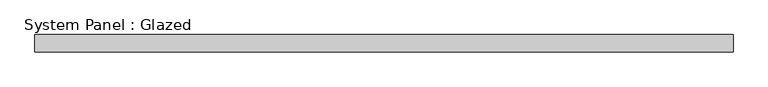
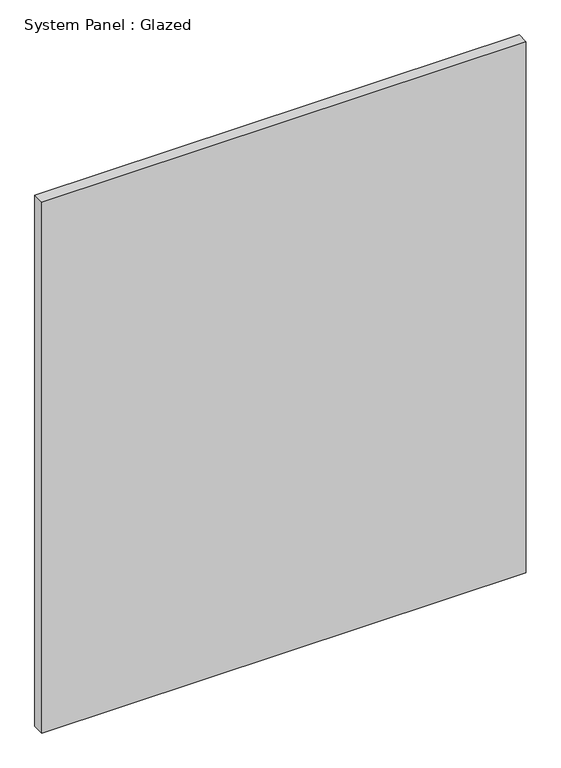
"""IFC4 building model written with IfcOpenShell, lengths in millimetres: plate geometry, System Panel : Glazed."""

from ifc_helpers import new_model, si_unit, origin, origin_with_axes, place, context, project, spatial, polyline, outline, extrude, source, transform, mapped, element, save


def system_panel_glazed_ec73f643(model_context):
    return source(origin(), model_context, "Body", "SweptSolid", [
        extrude(outline(polyline([(517.525, 19.05), (-517.525, 19.05), (-517.525, 44.45), (517.525, 44.45), (517.525, 19.05)])), origin_with_axes(), (0.0, 0.0, 1.0), 1198.6188597),
    ])


if __name__ == "__main__":
    model = new_model("IFC4")
    model_context = context("Model", 3, world=origin())
    ifc_project = project(units=[si_unit("LENGTHUNIT", "METRE", prefix="MILLI")], contexts=[model_context])
    site = spatial("IfcSite", under=ifc_project)
    building = spatial("IfcBuilding", under=site)
    placement = place(None, origin())
    system_panel_glazed_shape = system_panel_glazed_ec73f643(model_context)
    element("IfcPlate", 1, ObjectType="System Panel : Glazed", at=placement, inside=building, context=model_context, shape_type="MappedRepresentation", body=[
        mapped(system_panel_glazed_shape, transform((0.0, 0.0, 0.0), x_axis=(1.0, 0.0, 0.0), y_axis=(0.0, 1.0, 0.0), z_axis=(0.0, 0.0, 1.0))),
    ])
    save(model, "model.ifc")

# Revit data of these elements
# Type "System Panel : Glazed"
#   Construction Type Id = "GSP4R"
#   Analytic Construction = "1/8 in Pilkington single glazing"
#   Visual Light Transmittance = 0.9
#   Solar Heat Gain Coefficient = 0.86
#   Heat Transfer Coefficient (U) = 1.18115 BTU/(h·ft²·°F)
#   Define Thermal Properties by = 1
# Element 1 (IfcPlate, "System Panel : Glazed")
#   Materials on its faces: "Glass"
# Materials
#   "Glass": class "Glass", colour RGB 0 128 192, transparency 0.75, Description = "Soda Lime Glass", Cost = 0
